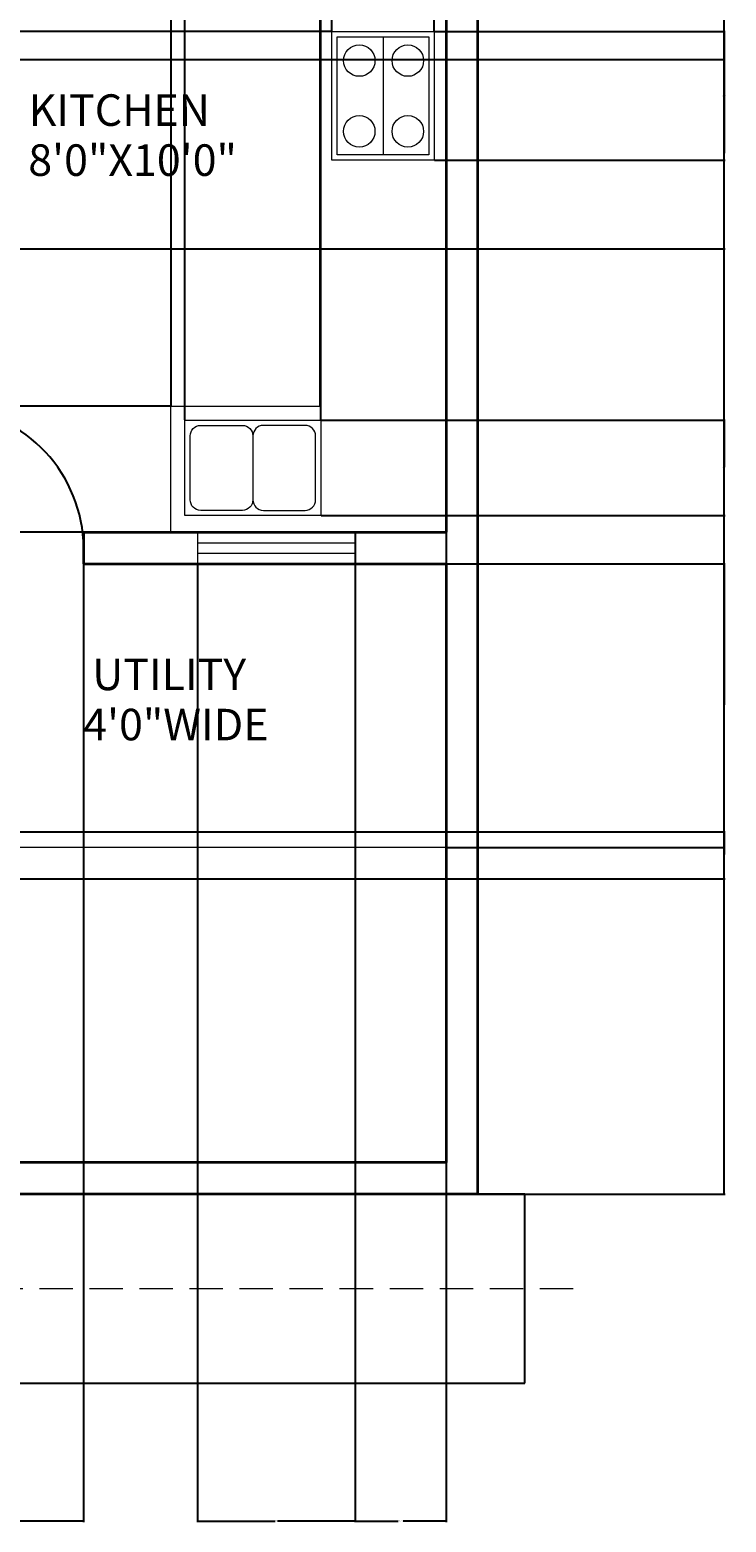
# Model space of a CAD drawing. Units: inches. Extents: x 2608 to 3003, y 1827 to 2396.
# Tile 2 of 5: x 2871 to 3003, y 1827 to 2111. Entities that reach past the tile are written whole.
import ezdxf

# ---------------------------------------------------------------- set-up
doc = ezdxf.new("R2010")
doc.units = ezdxf.units.IN
doc.linetypes.add('DASHED2', pattern=[9.525, 6.35, -3.175])
for name, color, linetype, lineweight in [('A-ANNO-DIMS', 2, 'Continuous', 18), ('A-AREA-IDEN', 7, 'Continuous', 25), ('A-DOOR', 50, 'Continuous', 25), ('A-EQPM', 213, 'Continuous', 18), ('A-FLOR', 111, 'Continuous', 18), ('A-FLOR-CASE', 213, 'Continuous', 18), ('A-FLOR-FIXT', 213, 'Continuous', 18), ('A-GLAZ', 40, 'Continuous', 18), ('A-WALL', 111, 'Continuous', 35), ('C-ROAD', 111, 'Continuous', 25), ('C-ROAD-CNTR', 255, 'DASHED2', 18)]:
    doc.layers.add(name, color=color, linetype=linetype, lineweight=lineweight)
doc.styles.get("Standard").update_dxf_attribs({"font": 'arial.ttf'})
doc.dimstyles.get("Standard").update_dxf_attribs({"dimtxt": 0.18, "dimasz": 0.18, "dimexe": 0.18, "dimexo": 0.0625, "dimgap": 0.09, "dimtad": 0, "dimtih": 1, "dimtoh": 1, "dimdec": 4, "dimzin": 0, "dimdsep": 46, "dimtxsty": 'Standard', "dimcen": 0.09, "dimadec": 0, "dimazin": 0, "dimtfac": 1, "dimtdec": 4, "dimtofl": 0, "dimtmove": 0, "dimatfit": 3, "dimfxl": 1, "dimtolj": 1, "dimtzin": 0, "dimarcsym": 0})

# ---------------------------------------------------------------- blocks, each defined once
blk = doc.blocks.new('*D29')
at = {"layer": 'A-ANNO-DIMS', "color": 0, "lineweight": -2, "transparency": 16777216}
for p, q in [((2955.98, 2369.49), (3003.02, 2369.49)), ((3002.84, 2369.31), (3002.84, 2129.67)), ((3002.84, 1889.67), (3002.84, 2129.31)), ((2955.98, 1889.49), (3003.02, 1889.49))]:
    blk.add_line(p, q, dxfattribs=at)
at = {"layer": 'A-ANNO-DIMS', "color": 0, "transparency": 16777216}
for points in [[(3002.81, 2369.31), (3002.87, 2369.31), (3002.84, 2369.49)], [(3002.81, 1889.67), (3002.87, 1889.67), (3002.84, 1889.49)]]:
    blk.add_solid(points, dxfattribs=at)
at = {"layer": 'Defpoints', "color": 0, "transparency": 16777216}
for p in [(2955.92, 2369.49), (3002.84, 2369.49), (2955.92, 1889.49)]:
    blk.add_point(p, dxfattribs=at)
at = {"layer": 'A-ANNO-DIMS', "color": 0, "transparency": 16777216, "insert": (3002.84, 2129.49), "char_height": 0.18, "attachment_point": 5}
blk.add_mtext('\\A1;480', dxfattribs=at)
blk = doc.blocks.new('*D51')
at = {"layer": 'A-ANNO-DIMS', "color": 0, "lineweight": -2, "transparency": 16777216}
for p, q in [((2853.92, 2009.43), (2853.92, 1827.03)), ((2880.92, 2009.43), (2880.92, 1827.03)), ((2854.1, 1827.21), (2867.2, 1827.21)), ((2880.74, 1827.21), (2867.64, 1827.21))]:
    blk.add_line(p, q, dxfattribs=at)
at = {"layer": 'A-ANNO-DIMS', "color": 0, "transparency": 16777216}
for points in [[(2854.1, 1827.24), (2854.1, 1827.18), (2853.92, 1827.21)], [(2880.74, 1827.24), (2880.74, 1827.18), (2880.92, 1827.21)]]:
    blk.add_solid(points, dxfattribs=at)
at = {"layer": 'Defpoints', "color": 0, "transparency": 16777216}
for p in [(2853.92, 2009.49), (2880.92, 2009.49), (2880.92, 1827.21)]:
    blk.add_point(p, dxfattribs=at)
at = {"layer": 'A-ANNO-DIMS', "color": 0, "transparency": 16777216, "insert": (2867.42, 1827.21), "char_height": 0.18, "attachment_point": 5}
blk.add_mtext('\\A1;27', dxfattribs=at)
blk = doc.blocks.new('*D52')
at = {"layer": 'A-ANNO-DIMS', "color": 0, "lineweight": -2, "transparency": 16777216}
for p, q in [((2902.61, 2009.43), (2902.61, 1827.03)), ((2932.61, 2009.43), (2932.61, 1827.03)), ((2902.79, 1827.21), (2917.39, 1827.21)), ((2932.43, 1827.21), (2917.83, 1827.21))]:
    blk.add_line(p, q, dxfattribs=at)
at = {"layer": 'A-ANNO-DIMS', "color": 0, "transparency": 16777216}
for points in [[(2902.79, 1827.24), (2902.79, 1827.18), (2902.61, 1827.21)], [(2932.43, 1827.24), (2932.43, 1827.18), (2932.61, 1827.21)]]:
    blk.add_solid(points, dxfattribs=at)
at = {"layer": 'Defpoints', "color": 0, "transparency": 16777216}
for p in [(2902.61, 2009.49), (2932.61, 2009.49), (2932.61, 1827.21)]:
    blk.add_point(p, dxfattribs=at)
at = {"layer": 'A-ANNO-DIMS', "color": 0, "transparency": 16777216, "insert": (2917.61, 1827.21), "char_height": 0.18, "attachment_point": 5}
blk.add_mtext('\\A1;30', dxfattribs=at)
blk = doc.blocks.new('*D53')
at = {"layer": 'A-ANNO-DIMS', "color": 0, "lineweight": -2, "transparency": 16777216}
for p, q in [((2932.61, 2015.43), (2932.61, 1827.03)), ((2949.92, 2015.43), (2949.92, 1827.03)), ((2932.79, 1827.21), (2940.81, 1827.21)), ((2949.74, 1827.21), (2941.72, 1827.21))]:
    blk.add_line(p, q, dxfattribs=at)
at = {"layer": 'A-ANNO-DIMS', "color": 0, "transparency": 16777216}
for points in [[(2932.79, 1827.24), (2932.79, 1827.18), (2932.61, 1827.21)], [(2949.74, 1827.24), (2949.74, 1827.18), (2949.92, 1827.21)]]:
    blk.add_solid(points, dxfattribs=at)
at = {"layer": 'Defpoints', "color": 0, "transparency": 16777216}
for p in [(2932.61, 2015.49), (2949.92, 2015.49), (2949.92, 1827.21)]:
    blk.add_point(p, dxfattribs=at)
at = {"layer": 'A-ANNO-DIMS', "color": 0, "transparency": 16777216, "insert": (2941.26, 1827.21), "char_height": 0.18, "attachment_point": 5}
blk.add_mtext('\\A1;17.305', dxfattribs=at)
blk = doc.blocks.new('*D56')
at = {"layer": 'A-ANNO-DIMS', "color": 0, "lineweight": -2, "transparency": 16777216}
for p, q in [((2897.48, 2039.49), (2607.92, 2039.49)), ((2608.1, 2039.31), (2608.1, 2027.67)), ((2608.1, 2015.67), (2608.1, 2027.31)), ((2897.48, 2015.49), (2607.92, 2015.49))]:
    blk.add_line(p, q, dxfattribs=at)
at = {"layer": 'A-ANNO-DIMS', "color": 0, "transparency": 16777216}
for points in [[(2608.07, 2039.31), (2608.13, 2039.31), (2608.1, 2039.49)], [(2608.07, 2015.67), (2608.13, 2015.67), (2608.1, 2015.49)]]:
    blk.add_solid(points, dxfattribs=at)
at = {"layer": 'Defpoints', "color": 0, "transparency": 16777216}
for p in [(2608.1, 2039.49), (2897.55, 2039.49), (2897.55, 2015.49)]:
    blk.add_point(p, dxfattribs=at)
at = {"layer": 'A-ANNO-DIMS', "color": 0, "transparency": 16777216, "insert": (2608.1, 2027.49), "char_height": 0.18, "attachment_point": 5}
blk.add_mtext('\\A1;24', dxfattribs=at)
blk = doc.blocks.new('*D57')
at = {"layer": 'A-ANNO-DIMS', "color": 0, "lineweight": -2, "transparency": 16777216}
for p, q in [((2897.55, 2039.55), (2897.55, 2395.95)), ((2897.73, 2395.77), (2911.34, 2395.77)), ((2925.74, 2395.77), (2912.13, 2395.77)), ((2925.92, 2039.55), (2925.92, 2395.95))]:
    blk.add_line(p, q, dxfattribs=at)
at = {"layer": 'A-ANNO-DIMS', "color": 0, "transparency": 16777216}
for points in [[(2897.73, 2395.8), (2897.73, 2395.74), (2897.55, 2395.77)], [(2925.74, 2395.8), (2925.74, 2395.74), (2925.92, 2395.77)]]:
    blk.add_solid(points, dxfattribs=at)
at = {"layer": 'Defpoints', "color": 0, "transparency": 16777216}
for p in [(2925.92, 2395.77), (2897.55, 2039.49), (2925.92, 2039.49)]:
    blk.add_point(p, dxfattribs=at)
at = {"layer": 'A-ANNO-DIMS', "color": 0, "transparency": 16777216, "insert": (2911.73, 2395.77), "char_height": 0.18, "attachment_point": 5}
blk.add_mtext('\\A1;28.37', dxfattribs=at)
blk = doc.blocks.new('*D59')
at = {"layer": 'A-ANNO-DIMS', "color": 0, "lineweight": -2, "transparency": 16777216}
for p, q in [((2949.98, 2009.49), (3003.02, 2009.49)), ((3002.84, 2009.31), (3002.84, 1982.67)), ((3002.84, 1955.67), (3002.84, 1982.31)), ((2949.98, 1955.49), (3003.02, 1955.49))]:
    blk.add_line(p, q, dxfattribs=at)
at = {"layer": 'A-ANNO-DIMS', "color": 0, "transparency": 16777216}
for points in [[(3002.81, 2009.31), (3002.87, 2009.31), (3002.84, 2009.49)], [(3002.81, 1955.67), (3002.87, 1955.67), (3002.84, 1955.49)]]:
    blk.add_solid(points, dxfattribs=at)
at = {"layer": 'Defpoints', "color": 0, "transparency": 16777216}
for p in [(2949.92, 2009.49), (3002.84, 2009.49), (2949.92, 1955.49)]:
    blk.add_point(p, dxfattribs=at)
at = {"layer": 'A-ANNO-DIMS', "color": 0, "transparency": 16777216, "insert": (3002.84, 1982.49), "char_height": 0.18, "attachment_point": 5}
blk.add_mtext('\\A1;54', dxfattribs=at)
blk = doc.blocks.new('*D60')
at = {"layer": 'A-ANNO-DIMS', "color": 0, "lineweight": -2, "transparency": 16777216}
for p, q in [((2928.16, 2110.88), (2928.16, 2395.95)), ((2928.34, 2395.77), (2937.45, 2395.77)), ((2947.47, 2395.77), (2938.36, 2395.77)), ((2947.65, 2110.88), (2947.65, 2395.95))]:
    blk.add_line(p, q, dxfattribs=at)
at = {"layer": 'A-ANNO-DIMS', "color": 0, "transparency": 16777216}
for points in [[(2928.34, 2395.8), (2928.34, 2395.74), (2928.16, 2395.77)], [(2947.47, 2395.8), (2947.47, 2395.74), (2947.65, 2395.77)]]:
    blk.add_solid(points, dxfattribs=at)
at = {"layer": 'Defpoints', "color": 0, "transparency": 16777216}
for p in [(2947.65, 2395.77), (2928.16, 2110.81), (2947.65, 2110.81)]:
    blk.add_point(p, dxfattribs=at)
at = {"layer": 'A-ANNO-DIMS', "color": 0, "transparency": 16777216, "insert": (2937.9, 2395.77), "char_height": 0.18, "attachment_point": 5}
blk.add_mtext('\\A1;19.493', dxfattribs=at)
blk = doc.blocks.new('*D61')
at = {"layer": 'A-ANNO-DIMS', "color": 0, "lineweight": -2, "transparency": 16777216}
for p, q in [((2947.71, 2110.81), (3003.02, 2110.81)), ((3002.84, 2110.63), (3002.84, 2098.76)), ((3002.84, 2086.51), (3002.84, 2098.39)), ((2947.71, 2086.33), (3003.02, 2086.33))]:
    blk.add_line(p, q, dxfattribs=at)
at = {"layer": 'A-ANNO-DIMS', "color": 0, "transparency": 16777216}
for points in [[(3002.81, 2110.63), (3002.87, 2110.63), (3002.84, 2110.81)], [(3002.81, 2086.51), (3002.87, 2086.51), (3002.84, 2086.33)]]:
    blk.add_solid(points, dxfattribs=at)
at = {"layer": 'Defpoints', "color": 0, "transparency": 16777216}
for p in [(2947.65, 2110.81), (3002.84, 2110.81), (2947.65, 2086.33)]:
    blk.add_point(p, dxfattribs=at)
at = {"layer": 'A-ANNO-DIMS', "color": 0, "transparency": 16777216, "insert": (3002.84, 2098.57), "char_height": 0.18, "attachment_point": 5}
blk.add_mtext('\\A1;24.48', dxfattribs=at)
blk = doc.blocks.new('*D62')
at = {"layer": 'A-ANNO-DIMS', "color": 0, "lineweight": -2, "transparency": 16777216}
for p, q in [((2925.85, 2135.49), (2607.92, 2135.49)), ((2608.1, 2135.31), (2608.1, 2123.33)), ((2608.1, 2110.99), (2608.1, 2122.97)), ((2928.1, 2110.81), (2607.92, 2110.81))]:
    blk.add_line(p, q, dxfattribs=at)
at = {"layer": 'A-ANNO-DIMS', "color": 0, "transparency": 16777216}
for points in [[(2608.07, 2135.31), (2608.13, 2135.31), (2608.1, 2135.49)], [(2608.07, 2110.99), (2608.13, 2110.99), (2608.1, 2110.81)]]:
    blk.add_solid(points, dxfattribs=at)
at = {"layer": 'Defpoints', "color": 0, "transparency": 16777216}
for p in [(2925.92, 2135.49), (2608.1, 2110.81), (2928.16, 2110.81)]:
    blk.add_point(p, dxfattribs=at)
at = {"layer": 'A-ANNO-DIMS', "color": 0, "transparency": 16777216, "insert": (2608.1, 2123.15), "char_height": 0.18, "attachment_point": 5}
blk.add_mtext('\\A1;24.675', dxfattribs=at)
blk = doc.blocks.new('*D63')
at = {"layer": 'A-ANNO-DIMS', "color": 0, "lineweight": -2, "transparency": 16777216}
for p, q in [((2900.2, 2036.91), (2900.2, 2395.95)), ((2900.38, 2395.77), (2912.67, 2395.77)), ((2925.89, 2395.77), (2913.6, 2395.77)), ((2926.07, 2036.91), (2926.07, 2395.95))]:
    blk.add_line(p, q, dxfattribs=at)
at = {"layer": 'A-ANNO-DIMS', "color": 0, "transparency": 16777216}
for points in [[(2900.38, 2395.8), (2900.38, 2395.74), (2900.2, 2395.77)], [(2925.89, 2395.8), (2925.89, 2395.74), (2926.07, 2395.77)]]:
    blk.add_solid(points, dxfattribs=at)
at = {"layer": 'Defpoints', "color": 0, "transparency": 16777216}
for p in [(2926.07, 2395.77), (2900.2, 2036.85), (2926.07, 2036.85)]:
    blk.add_point(p, dxfattribs=at)
at = {"layer": 'A-ANNO-DIMS', "color": 0, "transparency": 16777216, "insert": (2913.13, 2395.77), "char_height": 0.18, "attachment_point": 5}
blk.add_mtext('\\A1;25.865', dxfattribs=at)
blk = doc.blocks.new('*D64')
at = {"layer": 'A-ANNO-DIMS', "color": 0, "lineweight": -2, "transparency": 16777216}
for p, q in [((2926.13, 2036.85), (3003.02, 2036.85)), ((3002.84, 2036.67), (3002.84, 2027.94)), ((3002.84, 2018.85), (3002.84, 2027.58)), ((2926.13, 2018.67), (3003.02, 2018.67))]:
    blk.add_line(p, q, dxfattribs=at)
at = {"layer": 'A-ANNO-DIMS', "color": 0, "transparency": 16777216}
for points in [[(3002.81, 2036.67), (3002.87, 2036.67), (3002.84, 2036.85)], [(3002.81, 2018.85), (3002.87, 2018.85), (3002.84, 2018.67)]]:
    blk.add_solid(points, dxfattribs=at)
at = {"layer": 'Defpoints', "color": 0, "transparency": 16777216}
for p in [(2926.07, 2036.85), (3002.84, 2036.85), (2926.07, 2018.67)]:
    blk.add_point(p, dxfattribs=at)
at = {"layer": 'A-ANNO-DIMS', "color": 0, "transparency": 16777216, "insert": (3002.84, 2027.76), "char_height": 0.18, "attachment_point": 5}
blk.add_mtext('\\A1;18.176', dxfattribs=at)
blk = doc.blocks.new('*D66')
at = {"layer": 'A-ANNO-DIMS', "color": 0, "lineweight": -2, "transparency": 16777216}
for p, q in [((2691.98, 1958.49), (3003.02, 1958.49)), ((3002.84, 1958.31), (3002.84, 1954.17)), ((3002.84, 1949.67), (3002.84, 1953.81)), ((2691.98, 1949.49), (3003.02, 1949.49))]:
    blk.add_line(p, q, dxfattribs=at)
at = {"layer": 'A-ANNO-DIMS', "color": 0, "transparency": 16777216}
for points in [[(3002.81, 1958.31), (3002.87, 1958.31), (3002.84, 1958.49)], [(3002.81, 1949.67), (3002.87, 1949.67), (3002.84, 1949.49)]]:
    blk.add_solid(points, dxfattribs=at)
at = {"layer": 'Defpoints', "color": 0, "transparency": 16777216}
for p in [(2691.92, 1958.49), (3002.84, 1958.49), (2691.92, 1949.49)]:
    blk.add_point(p, dxfattribs=at)
at = {"layer": 'A-ANNO-DIMS', "color": 0, "transparency": 16777216, "insert": (3002.84, 1953.99), "char_height": 0.18, "attachment_point": 5}
blk.add_mtext('\\A1;9', dxfattribs=at)
blk = doc.blocks.new('*D68')
at = {"layer": 'A-ANNO-DIMS', "color": 0, "lineweight": -2, "transparency": 16777216}
for p, q in [((2736.98, 2105.49), (3003.02, 2105.49)), ((3002.84, 2105.31), (3002.84, 2087.67)), ((3002.84, 2069.67), (3002.84, 2087.31)), ((2736.98, 2069.49), (3003.02, 2069.49))]:
    blk.add_line(p, q, dxfattribs=at)
at = {"layer": 'A-ANNO-DIMS', "color": 0, "transparency": 16777216}
for points in [[(3002.81, 2105.31), (3002.87, 2105.31), (3002.84, 2105.49)], [(3002.81, 2069.67), (3002.87, 2069.67), (3002.84, 2069.49)]]:
    blk.add_solid(points, dxfattribs=at)
at = {"layer": 'Defpoints', "color": 0, "transparency": 16777216}
for p in [(2736.92, 2105.49), (3002.84, 2105.49), (2736.92, 2069.49)]:
    blk.add_point(p, dxfattribs=at)
at = {"layer": 'A-ANNO-DIMS', "color": 0, "transparency": 16777216, "insert": (3002.84, 2087.49), "char_height": 0.18, "attachment_point": 5}
blk.add_mtext('\\A1;36', dxfattribs=at)

msp = doc.modelspace()

# ---------------------------------------------------------------- linework, layer by layer
at = {"layer": 'A-DOOR'}
msp.add_arc((2853.9161, 2012.323), 27, 0.353483, 85.753071, dxfattribs=at)
at = {"layer": 'A-EQPM'}
msp.add_line((2937.9041, 2109.8146), (2937.9041, 2087.3341), dxfattribs=at)
for points in [[(2928.1576, 2110.8146), (2947.6506, 2110.8146), (2947.6506, 2086.3341), (2928.1576, 2086.3341)], [(2929.1576, 2109.8146), (2946.6506, 2109.8146), (2946.6506, 2087.3341), (2929.1576, 2087.3341)]]:
    msp.add_lwpolyline(points, close=True, dxfattribs=at)
for centre in [(2933.3773, 2105.3029), (2942.6298, 2105.3029), (2933.3773, 2091.8178), (2942.6298, 2091.8178)]:
    msp.add_circle(centre, 3, dxfattribs=at)
at = {"layer": 'A-FLOR'}
msp.add_line((2949.9155, 1955.4896), (2847.9155, 1955.4896), dxfattribs=at)
at = {"layer": 'A-FLOR-CASE'}
for p, q in [((2925.9155, 2135.4896), (2925.9155, 2039.4896)), ((2897.5458, 2015.4896), (2897.5458, 2039.4896)), ((2897.5458, 2039.4896), (2925.9155, 2039.4896))]:
    msp.add_line(p, q, dxfattribs=at)
at = {"layer": 'A-FLOR-FIXT'}
msp.add_lwpolyline([(2900.2006, 2036.8464), (2926.0657, 2036.8464), (2926.0657, 2018.6702), (2900.2006, 2018.6702)], close=True, dxfattribs=at)
msp.add_lwpolyline([(2913.1332, 2021.6702, -0.41421356), (2911.1332, 2019.6702), (2903.2006, 2019.6702, -0.41421356), (2901.2006, 2021.6702), (2901.2006, 2033.8464, -0.41421356), (2903.2006, 2035.8464), (2911.1332, 2035.8464, -0.41421356), (2913.1332, 2033.8464), (2913.1332, 2021.6702, 0.41421356), (2915.1332, 2019.6702), (2923.0657, 2019.6702, 0.41421356), (2925.0657, 2021.6702), (2925.0657, 2033.8464, 0.41421356), (2923.0657, 2035.8464), (2915.1332, 2035.8464, 0.41421356), (2913.1332, 2033.8464), (2913.1332, 2033.8464)], format="xyb", dxfattribs=at)
at = {"layer": 'A-GLAZ'}
for p, q in [((2902.6103, 2015.4896), (2902.6103, 2009.4896)), ((2932.6103, 2015.4896), (2932.6103, 2009.4896)), ((2902.6103, 2013.4896), (2932.6103, 2013.4896)), ((2902.6103, 2011.4896), (2932.6103, 2011.4896))]:
    msp.add_line(p, q, dxfattribs=at)
at = {"layer": 'A-WALL'}
for p, q in [((2949.9155, 2135.4896), (2949.9155, 2015.4896)), ((2880.9155, 2015.4896), (2880.9155, 2009.4896)), ((2880.9155, 2015.4896), (2949.9155, 2015.4896)), ((2880.9155, 2009.4896), (2949.9155, 2009.4896)), ((2949.9155, 2009.4896), (2949.9155, 1895.4896)), ((2949.9155, 1895.4896), (2805.9155, 1895.4896))]:
    msp.add_line(p, q, dxfattribs=at)
msp.add_lwpolyline([(2655.9155, 2369.4896), (2955.9155, 2369.4896), (2955.9155, 1889.4896), (2655.9155, 1889.4896)], close=True, dxfattribs=at)
at = {"layer": 'C-ROAD'}
for p, q in [((2964.9155, 1889.4896), (2955.9155, 1889.4896)), ((2964.9155, 1853.4896), (2964.9155, 1889.4896)), ((2646.9155, 1853.4896), (2964.9155, 1853.4896))]:
    msp.add_line(p, q, dxfattribs=at)
at = {"layer": 'C-ROAD-CNTR'}
msp.add_line((2634.3755, 1871.4896), (2976.5614, 1871.4896), dxfattribs=at)

# ---------------------------------------------------------------- texts
at = {"layer": 'A-AREA-IDEN'}
for tag, p in [('KITCHEN', (2870.4434, 2092.872)), ('8\'0"X10\'0"', (2870.3821, 2083.3515)), ('UTILITY', (2882.5609, 1985.4383)), ('4\'0"WIDE', (2880.8395, 1975.8832))]:
    msp.add_attdef(tag, p, '', height=6, dxfattribs=at)

# ---------------------------------------------------------------- dimensions: what is measured, and where the dimension line sits
at = {"layer": 'A-ANNO-DIMS'}
for base, p1, p2, override, picture, middle in [((2925.9155, 2395.7696), (2897.5458, 2039.4896), (2925.9155, 2039.4896), {"dimdec": 2, "dimlfac": 1, "dimrnd": 0, "dimzin": 0, "dimdsep": 46, "dimlunit": 2}, '*D57', (2911.7307, 2395.7696)), ((2926.0657, 2395.7696), (2900.2006, 2036.8464), (2926.0657, 2036.8464), {"dimdec": 3, "dimlfac": 1, "dimrnd": 0, "dimzin": 0, "dimdsep": 46, "dimlunit": 2}, '*D63', (2913.1332, 2395.7696)), ((2947.6506, 2395.7696), (2928.1576, 2110.8146), (2947.6506, 2110.8146), {"dimdec": 3, "dimlfac": 1, "dimrnd": 0, "dimzin": 0, "dimdsep": 46, "dimlunit": 2}, '*D60', (2937.9041, 2395.7696)), ((2949.9155, 1827.2096), (2932.6103, 2015.4896), (2949.9155, 2015.4896), {"dimdec": 3, "dimlfac": 1, "dimrnd": 0, "dimzin": 0, "dimdsep": 46, "dimlunit": 2}, '*D53', (2941.2629, 1827.2096)), ((2880.9155, 1827.2096), (2853.9155, 2009.4896), (2880.9155, 2009.4896), {"dimdec": 0, "dimlfac": 1, "dimrnd": 0, "dimzin": 0, "dimdsep": 46, "dimlunit": 2}, '*D51', (2867.4155, 1827.2096)), ((2932.6103, 1827.2096), (2902.6103, 2009.4896), (2932.6103, 2009.4896), {"dimdec": 0, "dimlfac": 1, "dimrnd": 0, "dimzin": 0, "dimdsep": 46, "dimlunit": 2}, '*D52', (2917.6103, 1827.2096))]:
    dim = msp.add_linear_dim(base=base, p1=p1, p2=p2, dimstyle='Standard', override=override, dxfattribs=at)
    dim.commit()
    dim.dimension.update_dxf_attribs({"geometry": picture, "text_midpoint": middle})
for base, p1, p2, override, picture, middle in [((3002.8414, 2369.4896), (2955.9155, 1889.4896), (2955.9155, 2369.4896), {"dimdec": 0, "dimlfac": 1, "dimrnd": 0, "dimzin": 0, "dimdsep": 46, "dimlunit": 2}, '*D29', (3002.8414, 2129.4896)), ((2608.0955, 2110.8146), (2925.9155, 2135.4896), (2928.1576, 2110.8146), {"dimdec": 3, "dimlfac": 1, "dimrnd": 0, "dimzin": 0, "dimdsep": 46, "dimlunit": 2}, '*D62', (2608.0955, 2123.1521)), ((3002.8414, 2110.8146), (2947.6506, 2086.3341), (2947.6506, 2110.8146), {"dimdec": 2, "dimlfac": 1, "dimrnd": 0, "dimzin": 0, "dimdsep": 46, "dimlunit": 2}, '*D61', (3002.8414, 2098.5743)), ((3002.8414, 2105.4896), (2736.9155, 2069.4896), (2736.9155, 2105.4896), {"dimdec": 0, "dimlfac": 1, "dimrnd": 0, "dimzin": 0, "dimdsep": 46, "dimlunit": 2}, '*D68', (3002.8414, 2087.4896)), ((2608.0955, 2039.4896), (2897.5458, 2015.4896), (2897.5458, 2039.4896), {"dimdec": 0, "dimlfac": 1, "dimrnd": 0, "dimzin": 0, "dimdsep": 46, "dimlunit": 2}, '*D56', (2608.0955, 2027.4896)), ((3002.8414, 2036.8464), (2926.0657, 2018.6702), (2926.0657, 2036.8464), {"dimdec": 3, "dimlfac": 1, "dimrnd": 0, "dimzin": 0, "dimdsep": 46, "dimlunit": 2}, '*D64', (3002.8414, 2027.7583)), ((3002.8414, 2009.4896), (2949.9155, 1955.4896), (2949.9155, 2009.4896), {"dimdec": 0, "dimlfac": 1, "dimrnd": 0, "dimzin": 0, "dimdsep": 46, "dimlunit": 2}, '*D59', (3002.8414, 1982.4896)), ((3002.8414, 1958.4896), (2691.9155, 1949.4896), (2691.9155, 1958.4896), {"dimdec": 0, "dimlfac": 1, "dimrnd": 0, "dimzin": 0, "dimdsep": 46, "dimlunit": 2}, '*D66', (3002.8414, 1953.9896))]:
    dim = msp.add_linear_dim(base=base, p1=p1, p2=p2, angle=90, dimstyle='Standard', override=override, dxfattribs=at)
    dim.commit()
    dim.dimension.update_dxf_attribs({"geometry": picture, "text_midpoint": middle})

doc.saveas('drawing.dxf')
